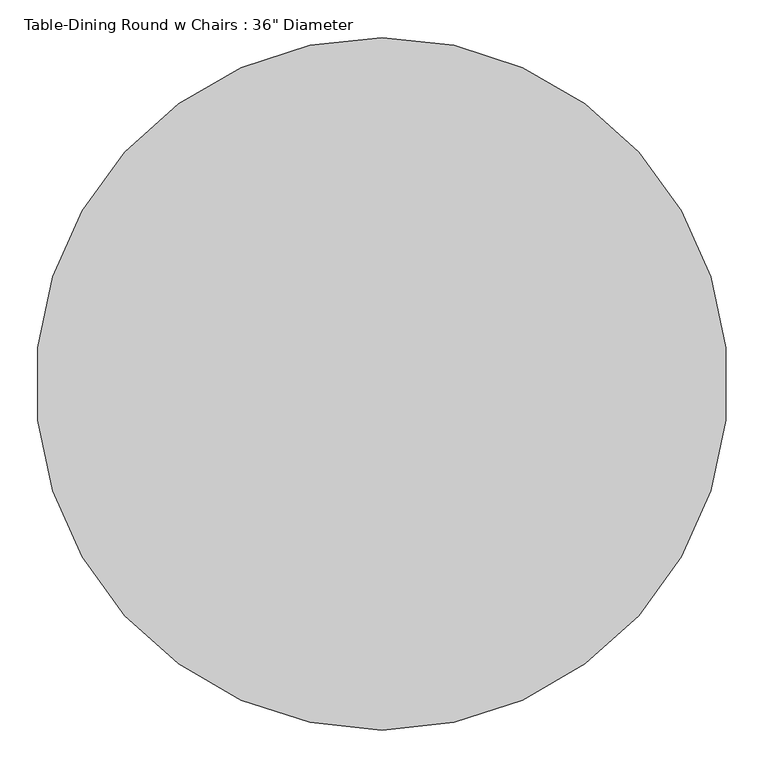
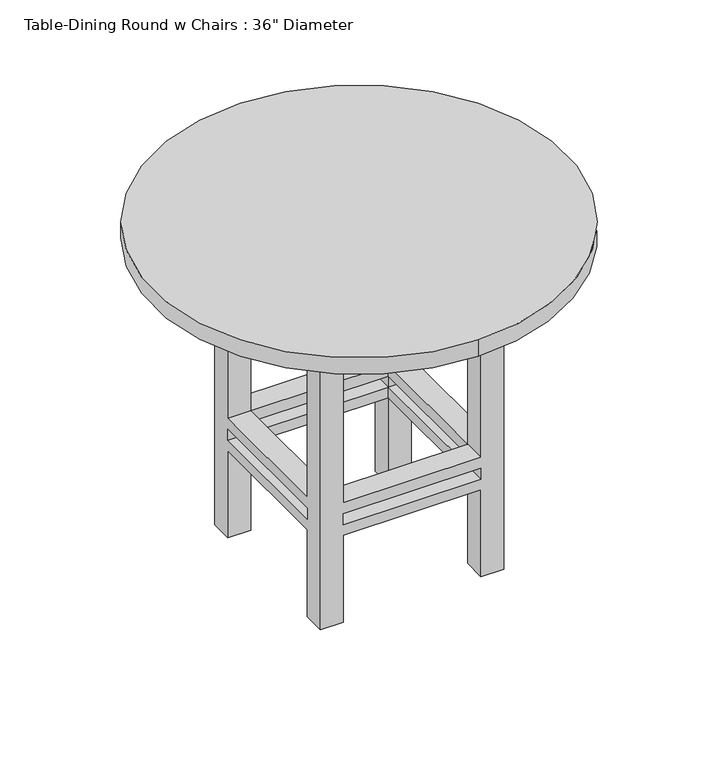
"""IFC4 building model written with IfcOpenShell, lengths in millimetres: furniture geometry."""

from ifc_helpers import new_model, si_unit, point, frame, frame_2d, origin, place, context, project, spatial, polyline, circle_curve, trimmed, segment, composite_curve, outline, extrude, faceted_brep, source, transform, mapped, element, save


def furniture_52f35bf4(model_context):
    return source(origin(), model_context, "Body", "SolidModel", [
        extrude(outline(polyline([(332.2819672, 43.7213115), (332.2819672, -413.4786885), (-124.9180328, -413.4786885), (-124.9180328, 43.7213115), (332.2819672, 43.7213115)]), holes=[polyline([(306.8819672, 18.3213115), (-99.5180328, 18.3213115), (-99.5180328, -388.0786885), (306.8819672, -388.0786885), (306.8819672, 18.3213115)])]), frame((0.0, 0.0, 647.7), z_axis=(0.0, 0.0, 1.0), x_axis=(1.0, 0.0, 0.0)), (0.0, 0.0, 1.0), 76.2),
        faceted_brep([(256.0819672, -32.4786885, 279.4), (256.0819672, -337.2786885, 279.4), (306.8819672, -337.2786885, 279.4), (306.8819672, -32.4786885, 279.4), (-48.7180328, -337.2786885, 279.4), (-48.7180328, -388.0786885, 279.4), (256.0819672, -388.0786885, 279.4), (-48.7180328, -32.4786885, 279.4), (-99.5180328, -32.4786885, 279.4), (-99.5180328, -337.2786885, 279.4), (256.0819672, 18.3213115, 279.4), (-48.7180328, 18.3213115, 279.4), (256.0819672, -32.4786885, 254.0), (-48.7180328, -32.4786885, 254.0), (-48.7180328, 18.3213115, 254.0), (256.0819672, 18.3213115, 254.0), (-48.7180328, -337.2786885, 254.0), (-99.5180328, -337.2786885, 254.0), (-99.5180328, -32.4786885, 254.0), (256.0819672, -337.2786885, 254.0), (256.0819672, -388.0786885, 254.0), (-48.7180328, -388.0786885, 254.0), (306.8819672, -32.4786885, 254.0), (306.8819672, -337.2786885, 254.0), (-99.5180328, 18.3213115, 647.7), (-48.7180328, 18.3213115, 647.7), (256.0819672, 18.3213115, 647.7), (306.8819672, 18.3213115, 647.7), (306.8819672, 18.3213115, 0.0), (256.0819672, 18.3213115, 0.0), (256.0819672, 18.3213115, 203.2), (-48.7180328, 18.3213115, 203.2), (-48.7180328, 18.3213115, 0.0), (-99.5180328, 18.3213115, 0.0), (-48.7180328, 18.3213115, 228.6), (256.0819672, 18.3213115, 228.6), (-99.5180328, -32.4786885, 647.7), (-99.5180328, -32.4786885, 0.0), (-99.5180328, -32.4786885, 203.2), (-99.5180328, -337.2786885, 203.2), (-99.5180328, -337.2786885, 0.0), (-99.5180328, -388.0786885, 0.0), (-99.5180328, -388.0786885, 647.7), (-99.5180328, -337.2786885, 647.7), (-99.5180328, -337.2786885, 228.6), (-99.5180328, -32.4786885, 228.6), (306.8819672, -388.0786885, 647.7), (256.0819672, -388.0786885, 647.7), (-48.7180328, -388.0786885, 647.7), (-48.7180328, -388.0786885, 0.0), (-48.7180328, -388.0786885, 203.2), (256.0819672, -388.0786885, 203.2), (256.0819672, -388.0786885, 0.0), (306.8819672, -388.0786885, 0.0), (256.0819672, -388.0786885, 228.6), (-48.7180328, -388.0786885, 228.6), (306.8819672, -32.4786885, 647.7), (306.8819672, -337.2786885, 647.7), (306.8819672, -337.2786885, 0.0), (306.8819672, -337.2786885, 203.2), (306.8819672, -32.4786885, 203.2), (306.8819672, -32.4786885, 0.0), (306.8819672, -32.4786885, 228.6), (306.8819672, -337.2786885, 228.6), (-48.7180328, -32.4786885, 647.7), (256.0819672, -337.2786885, 647.7), (256.0819672, -32.4786885, 647.7), (-48.7180328, -337.2786885, 647.7), (256.0819672, -32.4786885, 0.0), (-48.7180328, -337.2786885, 0.0), (-48.7180328, -32.4786885, 0.0), (256.0819672, -337.2786885, 0.0), (-48.7180328, -32.4786885, 228.6), (-48.7180328, -32.4786885, 203.2), (256.0819672, -32.4786885, 228.6), (256.0819672, -32.4786885, 203.2), (256.0819672, -337.2786885, 228.6), (256.0819672, -337.2786885, 203.2), (-48.7180328, -337.2786885, 228.6), (-48.7180328, -337.2786885, 203.2)], [[[0, 1, 2, 3]], [[1, 4, 5, 6]], [[4, 7, 8, 9]], [[7, 0, 10, 11]], [[12, 13, 14, 15]], [[13, 16, 17, 18]], [[16, 19, 20, 21]], [[19, 12, 22, 23]], [[24, 25, 11, 10, 26, 27, 28, 29, 30, 31, 32, 33], [14, 34, 35, 15]], [[36, 24, 33, 37, 38, 39, 40, 41, 42, 43, 9, 8], [17, 44, 45, 18]], [[46, 47, 6, 5, 48, 42, 41, 49, 50, 51, 52, 53], [20, 54, 55, 21]], [[28, 27, 56, 3, 2, 57, 46, 53, 58, 59, 60, 61], [22, 62, 63, 23]], [[1, 0, 12, 19]], [[4, 1, 19, 16]], [[7, 4, 16, 13]], [[0, 7, 13, 12]], [[25, 24, 36, 64]], [[47, 46, 57, 65]], [[26, 66, 56, 27]], [[48, 67, 43, 42]], [[29, 28, 61, 68]], [[49, 41, 40, 69]], [[32, 70, 37, 33]], [[52, 71, 58, 53]], [[13, 18, 45, 72]], [[64, 36, 8, 7]], [[37, 70, 73, 38]], [[14, 13, 72, 34]], [[25, 64, 7, 11]], [[70, 32, 31, 73]], [[12, 15, 35, 74]], [[66, 26, 10, 0]], [[29, 68, 75, 30]], [[22, 12, 74, 62]], [[56, 66, 0, 3]], [[68, 61, 60, 75]], [[19, 23, 63, 76]], [[65, 57, 2, 1]], [[58, 71, 77, 59]], [[20, 19, 76, 54]], [[47, 65, 1, 6]], [[71, 52, 51, 77]], [[16, 21, 55, 78]], [[67, 48, 5, 4]], [[49, 69, 79, 50]], [[17, 16, 78, 44]], [[43, 67, 4, 9]], [[69, 40, 39, 79]], [[74, 76, 63, 62]], [[76, 78, 55, 54]], [[78, 72, 45, 44]], [[72, 74, 35, 34]], [[75, 73, 31, 30]], [[73, 79, 39, 38]], [[79, 77, 51, 50]], [[77, 75, 60, 59]], [[76, 74, 75, 77]], [[78, 76, 77, 79]], [[72, 78, 79, 73]], [[74, 72, 73, 75]]]),
        extrude(outline(composite_curve([segment(trimmed(circle_curve(frame_2d((103.6819672, -184.8786885)), 457.2), [point((103.6819672, -642.0786885))], [point((103.6819672, 272.3213115))], False, "CARTESIAN"), True, "CONTINUOUS"), segment(trimmed(circle_curve(frame_2d((103.6819672, -184.8786885)), 457.2), [point((103.6819672, 272.3213115))], [point((103.6819672, -642.0786885))], False, "CARTESIAN"), True, "CONTINUOUS")], self_intersect=False)), frame((0.0, 0.0, 723.9), z_axis=(0.0, 0.0, 1.0), x_axis=(1.0, 0.0, 0.0)), (0.0, 0.0, 1.0), 38.1),
    ])


if __name__ == "__main__":
    model = new_model("IFC4")
    model_context = context("Model", 3, world=origin())
    ifc_project = project(units=[si_unit("LENGTHUNIT", "METRE", prefix="MILLI")], contexts=[model_context])
    site = spatial("IfcSite", under=ifc_project)
    building = spatial("IfcBuilding", under=site)
    placement = place(None, origin())
    furniture_shape = furniture_52f35bf4(model_context)
    element("IfcFurniture", 1, ObjectType="Table-Dining Round w Chairs : 36\" Diameter", at=placement, inside=building, context=model_context, shape_type="MappedRepresentation", body=[
        mapped(furniture_shape, transform((0.0, 0.0, 0.0), x_axis=(1.0, 0.0, 0.0), y_axis=(0.0, 1.0, 0.0), z_axis=(0.0, 0.0, 1.0))),
    ])
    save(model, "model.ifc")

# Revit data of these elements
# Type "Table-Dining Round w Chairs : 36\" Diameter"
#   Assembly Code = "E2020200"
#   Radius = 1' - 6"
#   Diameter = 3' - 0"
#   Height = 2' - 6"
#   Chairs = 4
#   Base Material = Pine
#   Top Material = Laminate, Linen, Matte
#   Default Elevation = 0
# Element 1 (IfcFurniture, "Table-Dining Round w Chairs : 36\" Diameter")
#   Materials on its faces: "Pine", "Laminate, Linen, Matte"
# Materials
#   "Pine": class "Wood", colour RGB 223 192 134, transparency 0, Description = "Pinus Echinata", Cost = 0
#   "Laminate, Linen, Matte": class "Plastic", colour RGB 249 239 230, transparency 0, Description = "Plastic Laminate - Linen, Matte", Cost = 0
